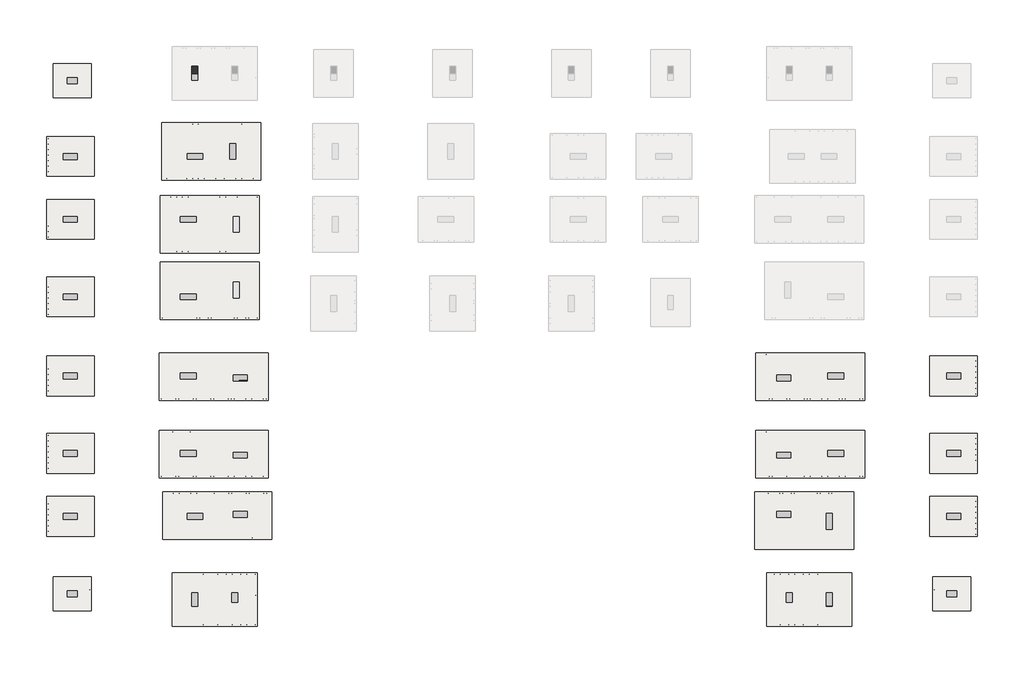
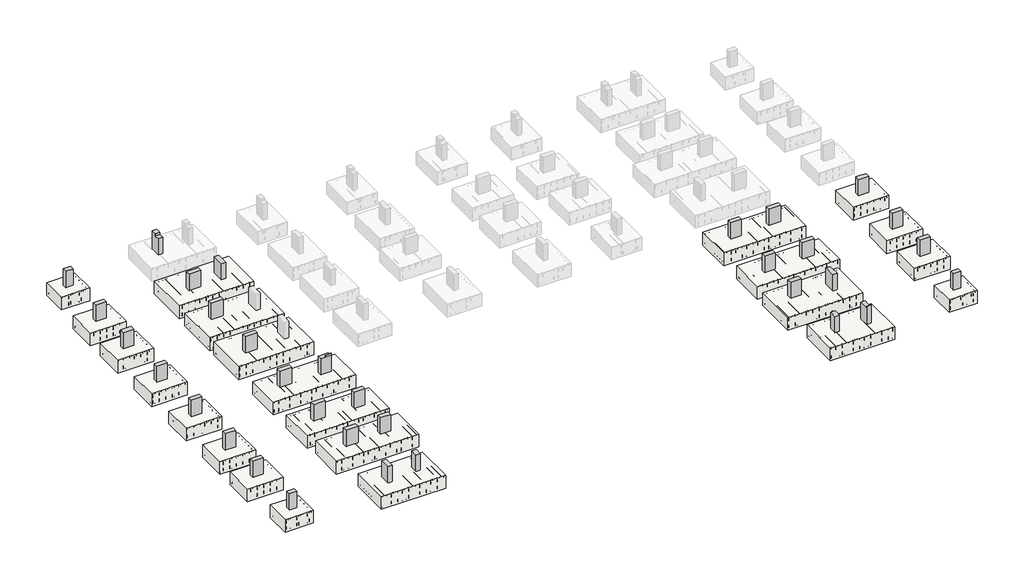
# One storey, part 1 of 21: 33 columns, 23 slabs.
"""IFC4 building model written with IfcOpenShell, lengths in millimetres."""

from ifc_helpers import new_model, si_unit, frame, origin, place, context, project, spatial, polyline, outline, extrude, faceted_brep, transform, mapped, element, save
from components import m_footing_rectangular_1900x1700x900_f1_617558a1, m_footing_rectangular_2400x2000x900_f2_ceb4d106, m_footing_rectangular_2700x4300x900_f4_c3563192, m_footing_rectangular_5000x2900x900_f5_2a8e231f, m_footing_rectangular_5500x2400x900_f6_6a8cdcd2

model = new_model("IFC4")

# Units and contexts
model_context = context("Model", 3, world=origin())
ifc_project = project(units=[si_unit("LENGTHUNIT", "METRE", prefix="MILLI")], contexts=[model_context])

# Site, building, storey
site = spatial("IfcSite", under=ifc_project)
building = spatial("IfcBuilding", under=site)
storey = spatial("IfcBuildingStorey", under=building, Elevation=-1100.0)

# Columns
placement = place(None, origin())
element("IfcColumn", 1, ObjectType="M_Concrete-Rectangular-Column : 300X500 C1", at=placement, inside=storey, context=model_context, shape_type="Brep", body=[
    faceted_brep([(-24350.8326863, 14604.1704288, -1100.0), (-23850.8326863, 14604.1704288, -1100.0), (-23850.8326863, 14304.1704288, -1100.0), (-24350.8326863, 14304.1704288, -1100.0), (-24350.8326863, 14604.1704288, 50.0), (-23850.8326863, 14604.1704288, 50.0), (-23850.8326863, 14304.1704288, 50.0), (-24150.8326863, 14304.1704288, 50.0), (-24350.8326863, 14304.1704288, 50.0)], [[[0, 1, 2, 3]], [[1, 0, 4, 5]], [[2, 1, 5, 6]], [[3, 2, 6, 7, 8]], [[0, 3, 8, 4]], [[5, 4, 8, 7, 6]]]),
])
element("IfcColumn", 2, ObjectType="M_Concrete-Rectangular-Column : 300X500 C1", at=placement, inside=storey, context=model_context, shape_type="Brep", body=[
    faceted_brep([(-24350.8326863, -11305.8295712, -1100.0), (-23850.8326863, -11305.8295712, -1100.0), (-23850.8326863, -11605.8295712, -1100.0), (-24350.8326863, -11605.8295712, -1100.0), (-24350.8326863, -11305.8295712, 50.0), (-24150.8326863, -11305.8295712, 50.0), (-23850.8326863, -11305.8295712, 50.0), (-23850.8326863, -11605.8295712, 50.0), (-24350.8326863, -11605.8295712, 50.0)], [[[0, 1, 2, 3]], [[1, 0, 4, 5, 6]], [[2, 1, 6, 7]], [[3, 2, 7, 8]], [[0, 3, 8, 4]], [[6, 5, 4, 8, 7]]]),
])
element("IfcColumn", 3, ObjectType="M_Concrete-Rectangular-Column : 300X500 C1", at=placement, inside=storey, context=model_context, shape_type="Brep", body=[
    faceted_brep([(20029.1673137, -11305.8295712, -1100.0), (20529.1673137, -11305.8295712, -1100.0), (20529.1673137, -11605.8295712, -1100.0), (20029.1673137, -11605.8295712, -1100.0), (20029.1673137, -11305.8295712, 50.0), (20329.1673137, -11305.8295712, 50.0), (20529.1673137, -11305.8295712, 50.0), (20529.1673137, -11605.8295712, 50.0), (20029.1673137, -11605.8295712, 50.0)], [[[0, 1, 2, 3]], [[1, 0, 4, 5, 6]], [[2, 1, 6, 7]], [[3, 2, 7, 8]], [[0, 3, 8, 4]], [[6, 5, 4, 8, 7]]]),
])
element("IfcColumn", 4, ObjectType="M_Concrete-Rectangular-Column : 300X500 C1", at=placement, inside=storey, context=model_context, shape_type="Brep", body=[
    faceted_brep([(11939.1673137, -11895.8295712, -1100.0), (11939.1673137, -11395.8295712, -1100.0), (12239.1673137, -11395.8295712, -1100.0), (12239.1673137, -11895.8295712, -1100.0), (11939.1673137, -11895.8295712, 50.0), (11939.1673137, -11395.8295712, 50.0), (12239.1673137, -11395.8295712, 50.0), (12239.1673137, -11695.8295712, 50.0), (12239.1673137, -11895.8295712, 50.0)], [[[0, 1, 2, 3]], [[1, 0, 4, 5]], [[2, 1, 5, 6]], [[3, 2, 6, 7, 8]], [[0, 3, 8, 4]], [[5, 4, 8, 7, 6]]]),
])
element("IfcColumn", 5, ObjectType="M_Concrete-Rectangular-Column : 300X500 C1", at=placement, inside=storey, context=model_context, shape_type="Brep", body=[
    faceted_brep([(-16061.8300669, -11895.8295712, -1100.0), (-16061.8300669, -11395.8295712, -1100.0), (-15761.8300669, -11395.8295712, -1100.0), (-15761.8300669, -11895.8295712, -1100.0), (-16061.8300669, -11895.8295712, 50.0), (-16061.8300669, -11695.8295712, 50.0), (-16061.8300669, -11395.8295712, 50.0), (-15761.8300669, -11395.8295712, 50.0), (-15761.8300669, -11895.8295712, 50.0)], [[[0, 1, 2, 3]], [[1, 0, 4, 5, 6]], [[2, 1, 6, 7]], [[3, 2, 7, 8]], [[0, 3, 8, 4]], [[6, 5, 4, 8, 7]]]),
])
element("IfcColumn", 6, ObjectType="M_Concrete-Rectangular-Column : 300X700 C2", at=placement, inside=storey, context=model_context, shape_type="Brep", body=[
    faceted_brep([(-17760.8326863, 15184.1704288, -1100.0), (-17760.8326863, 14484.1704288, -1100.0), (-18060.8326863, 14484.1704288, -1100.0), (-18060.8326863, 15184.1704288, -1100.0), (-17760.8326863, 15184.1704288, 200.0), (-17760.8326863, 14806.5875097, 200.0), (-17760.8326863, 14806.5875097, 50.0), (-17760.8326863, 14484.1704288, 50.0), (-18060.8326863, 14484.1704288, 50.0), (-18060.8326863, 14806.3616842, 50.0), (-18060.8326863, 14806.3616842, 200.0), (-18060.8326863, 15184.1704288, 200.0), (-18054.3658896, 14806.5875097, 200.0), (-18054.3658896, 14806.5875097, 50.0)], [[[0, 1, 2, 3]], [[1, 0, 4, 5, 6, 7]], [[2, 1, 7, 8]], [[3, 2, 8, 9, 10, 11]], [[0, 3, 11, 4]], [[4, 11, 10, 12, 5]], [[6, 13, 9, 8, 7]], [[13, 12, 10, 9]], [[12, 13, 6, 5]]]),
])
element("IfcColumn", 7, ObjectType="M_Concrete-Rectangular-Column : 300X700 C2", at=placement, inside=storey, context=model_context, shape_type="Brep", body=[
    faceted_brep([(-24550.8326863, 7604.1704288, -1100.0), (-23850.8326863, 7604.1704288, -1100.0), (-23850.8326863, 7304.1704288, -1100.0), (-24550.8326863, 7304.1704288, -1100.0), (-24550.8326863, 7604.1704288, 50.0), (-24150.8326863, 7604.1704288, 50.0), (-23850.8326863, 7604.1704288, 50.0), (-23850.8326863, 7604.1704288, -400.0), (-23850.8326863, 7304.1704288, 50.0), (-23850.8326863, 7304.1704288, -400.0), (-24150.8326863, 7304.1704288, 50.0), (-24550.8326863, 7304.1704288, 50.0)], [[[0, 1, 2, 3]], [[1, 0, 4, 5, 6, 7]], [[2, 1, 7, 6, 8, 9]], [[3, 2, 9, 8, 10, 11]], [[0, 3, 11, 4]], [[6, 5, 4, 11, 10, 8]]]),
])
element("IfcColumn", 8, ObjectType="M_Concrete-Rectangular-Column : 300X700 C2", at=placement, inside=storey, context=model_context, shape_type="Brep", body=[
    faceted_brep([(-24550.8326863, 3694.1704288, -1100.0), (-23850.8326863, 3694.1704288, -1100.0), (-23850.8326863, 3394.1704288, -1100.0), (-24550.8326863, 3394.1704288, -1100.0), (-24550.8326863, 3694.1704288, 50.0), (-24150.8326863, 3694.1704288, 50.0), (-23850.8326863, 3694.1704288, 50.0), (-23850.8326863, 3694.1704288, -400.0), (-23850.8326863, 3394.1704288, 50.0), (-23850.8326863, 3394.1704288, -400.0), (-24150.8326863, 3394.1704288, 50.0), (-24550.8326863, 3394.1704288, 50.0)], [[[0, 1, 2, 3]], [[1, 0, 4, 5, 6, 7]], [[2, 1, 7, 6, 8, 9]], [[3, 2, 9, 8, 10, 11]], [[0, 3, 11, 4]], [[6, 5, 4, 11, 10, 8]]]),
])
element("IfcColumn", 9, ObjectType="M_Concrete-Rectangular-Column : 300X700 C2", at=placement, inside=storey, context=model_context, shape_type="Brep", body=[
    faceted_brep([(-24550.8326863, -305.8295712, -1100.0), (-23850.8326863, -305.8295712, -1100.0), (-23850.8326863, -605.8295712, -1100.0), (-24550.8326863, -605.8295712, -1100.0), (-24550.8326863, -305.8295712, 50.0), (-24150.8326863, -305.8295712, 50.0), (-23850.8326863, -305.8295712, 50.0), (-23850.8326863, -305.8295712, -400.0), (-23850.8326863, -605.8295712, 50.0), (-23850.8326863, -605.8295712, -400.0), (-24150.8326863, -605.8295712, 50.0), (-24550.8326863, -605.8295712, 50.0)], [[[0, 1, 2, 3]], [[1, 0, 4, 5, 6, 7]], [[2, 1, 7, 6, 8, 9]], [[3, 2, 9, 8, 10, 11]], [[0, 3, 11, 4]], [[6, 5, 4, 11, 10, 8]]]),
])
element("IfcColumn", 10, ObjectType="M_Concrete-Rectangular-Column : 300X700 C2", at=placement, inside=storey, context=model_context, shape_type="Brep", body=[
    faceted_brep([(-24550.8326863, -4215.8295712, -1100.0), (-23850.8326863, -4215.8295712, -1100.0), (-23850.8326863, -4515.8295712, -1100.0), (-24550.8326863, -4515.8295712, -1100.0), (-24550.8326863, -4215.8295712, 50.0), (-24150.8326863, -4215.8295712, 50.0), (-23850.8326863, -4215.8295712, 50.0), (-23850.8326863, -4215.8295712, -400.0), (-23850.8326863, -4515.8295712, 50.0), (-23850.8326863, -4515.8295712, -400.0), (-24150.8326863, -4515.8295712, 50.0), (-24550.8326863, -4515.8295712, 50.0)], [[[0, 1, 2, 3]], [[1, 0, 4, 5, 6, 7]], [[2, 1, 7, 6, 8, 9]], [[3, 2, 9, 8, 10, 11]], [[0, 3, 11, 4]], [[6, 5, 4, 11, 10, 8]]]),
])
element("IfcColumn", 11, ObjectType="M_Concrete-Rectangular-Column : 300X700 C2", at=placement, inside=storey, context=model_context, shape_type="Brep", body=[
    faceted_brep([(-24550.8326863, -7395.8295712, -1100.0), (-23850.8326863, -7395.8295712, -1100.0), (-23850.8326863, -7695.8295712, -1100.0), (-24550.8326863, -7695.8295712, -1100.0), (-24550.8326863, -7395.8295712, 50.0), (-24150.8326863, -7395.8295712, 50.0), (-23850.8326863, -7395.8295712, 50.0), (-23850.8326863, -7395.8295712, -400.0), (-23850.8326863, -7695.8295712, 50.0), (-23850.8326863, -7695.8295712, -400.0), (-24150.8326863, -7695.8295712, 50.0), (-24550.8326863, -7695.8295712, 50.0)], [[[0, 1, 2, 3]], [[1, 0, 4, 5, 6, 7]], [[2, 1, 7, 6, 8, 9]], [[3, 2, 9, 8, 10, 11]], [[0, 3, 11, 4]], [[6, 5, 4, 11, 10, 8]]]),
])
element("IfcColumn", 12, ObjectType="M_Concrete-Rectangular-Column : 300X700 C2", at=placement, inside=storey, context=model_context, shape_type="Brep", body=[
    faceted_brep([(-18060.8326863, -12095.8295712, -1100.0), (-18060.8326863, -11395.8295712, -1100.0), (-17760.8326863, -11395.8295712, -1100.0), (-17760.8326863, -12095.8295712, -1100.0), (-18060.8326863, -12095.8295712, 50.0), (-18060.8326863, -11691.586009, 50.0), (-18060.8326863, -11395.8295712, 50.0), (-17760.8326863, -11395.8295712, 50.0), (-17760.8326863, -11695.8295712, 50.0), (-17760.8326863, -12095.8295712, 50.0)], [[[0, 1, 2, 3]], [[1, 0, 4, 5, 6]], [[2, 1, 6, 7]], [[3, 2, 7, 8, 9]], [[0, 3, 9, 4]], [[6, 5, 4, 9, 8, 7]]]),
])
element("IfcColumn", 13, ObjectType="M_Concrete-Rectangular-Column : 300X700 C2", at=placement, inside=storey, context=model_context, shape_type="Brep", body=[
    faceted_brep([(-15270.8326863, -7605.8295712, -1100.0), (-15970.8326863, -7605.8295712, -1100.0), (-15970.8326863, -7305.8295712, -1100.0), (-15270.8326863, -7305.8295712, -1100.0), (-15270.8326863, -7605.8295712, 50.0), (-15670.8326863, -7605.8295712, 50.0), (-15970.8326863, -7605.8295712, 50.0), (-15970.8326863, -7305.8295712, 50.0), (-15670.8326863, -7305.8295712, 50.0), (-15270.8326863, -7305.8295712, 50.0)], [[[0, 1, 2, 3]], [[1, 0, 4, 5, 6]], [[2, 1, 6, 7]], [[3, 2, 7, 8, 9]], [[0, 3, 9, 4]], [[6, 5, 4, 9, 8, 7]]]),
])
element("IfcColumn", 14, ObjectType="M_Concrete-Rectangular-Column : 300X700 C2", at=placement, inside=storey, context=model_context, shape_type="Brep", body=[
    faceted_brep([(-15270.8326863, -4605.8295712, -1100.0), (-15970.8326863, -4605.8295712, -1100.0), (-15970.8326863, -4305.8295712, -1100.0), (-15270.8326863, -4305.8295712, -1100.0), (-15270.8326863, -4605.8295712, 50.0), (-15670.8326863, -4605.8295712, 50.0), (-15970.8326863, -4605.8295712, 50.0), (-15970.8326863, -4605.8295712, -400.0), (-15970.8326863, -4305.8295712, 50.0), (-15970.8326863, -4305.8295712, -400.0), (-15670.8326863, -4305.8295712, 50.0), (-15270.8326863, -4305.8295712, 50.0)], [[[0, 1, 2, 3]], [[1, 0, 4, 5, 6, 7]], [[2, 1, 7, 6, 8, 9]], [[3, 2, 9, 8, 10, 11]], [[0, 3, 11, 4]], [[6, 5, 4, 11, 10, 8]]]),
])
element("IfcColumn", 15, ObjectType="M_Concrete-Rectangular-Column : 300X700 C2", at=placement, inside=storey, context=model_context, shape_type="Brep", body=[
    faceted_brep([(-15270.8326863, -695.8295712, -1100.0), (-15970.8326863, -695.8295712, -1100.0), (-15970.8326863, -395.8295712, -1100.0), (-15270.8326863, -395.8295712, -1100.0), (-15270.8326863, -695.8295712, 200.0), (-15670.8326863, -695.8295712, 200.0), (-15670.8326863, -695.8295712, 50.0), (-15970.8326863, -695.8295712, 50.0), (-15970.8326863, -695.8295712, -400.0), (-15970.8326863, -395.8295712, 50.0), (-15970.8326863, -395.8295712, -400.0), (-15270.8326863, -395.8295712, 50.0), (-15270.8326863, -693.8316044, 50.0), (-15270.8326863, -693.8316044, 200.0), (-15670.8326863, -693.8316044, 200.0), (-15670.8326863, -693.8316044, 50.0)], [[[0, 1, 2, 3]], [[1, 0, 4, 5, 6, 7, 8]], [[2, 1, 8, 7, 9, 10]], [[3, 2, 10, 9, 11]], [[0, 3, 11, 12, 13, 4]], [[4, 13, 14, 5]], [[15, 12, 11, 9, 7, 6]], [[12, 15, 14, 13]], [[14, 15, 6, 5]]]),
])
element("IfcColumn", 16, ObjectType="M_Concrete-Rectangular-Column : 300X700 C2", at=placement, inside=storey, context=model_context, shape_type="Brep", body=[
    faceted_brep([(20029.1673137, -305.8295712, -1100.0), (20729.1673137, -305.8295712, -1100.0), (20729.1673137, -605.8295712, -1100.0), (20029.1673137, -605.8295712, -1100.0), (20029.1673137, -305.8295712, -400.0), (20029.1673137, -305.8295712, 50.0), (20329.1673137, -305.8295712, 50.0), (20729.1673137, -305.8295712, 50.0), (20729.1673137, -605.8295712, 50.0), (20329.1673137, -605.8295712, 50.0), (20029.1673137, -605.8295712, 50.0), (20029.1673137, -605.8295712, -400.0)], [[[0, 1, 2, 3]], [[1, 0, 4, 5, 6, 7]], [[2, 1, 7, 8]], [[3, 2, 8, 9, 10, 11]], [[0, 3, 11, 10, 5, 4]], [[7, 6, 5, 10, 9, 8]]]),
])
element("IfcColumn", 17, ObjectType="M_Concrete-Rectangular-Column : 300X700 C2", at=placement, inside=storey, context=model_context, shape_type="Brep", body=[
    faceted_brep([(20029.1673137, -4215.8295712, -1100.0), (20729.1673137, -4215.8295712, -1100.0), (20729.1673137, -4515.8295712, -1100.0), (20029.1673137, -4515.8295712, -1100.0), (20029.1673137, -4215.8295712, -400.0), (20029.1673137, -4215.8295712, 50.0), (20329.1673137, -4215.8295712, 50.0), (20729.1673137, -4215.8295712, 50.0), (20729.1673137, -4515.8295712, 50.0), (20329.1673137, -4515.8295712, 50.0), (20029.1673137, -4515.8295712, 50.0), (20029.1673137, -4515.8295712, -400.0)], [[[0, 1, 2, 3]], [[1, 0, 4, 5, 6, 7]], [[2, 1, 7, 8]], [[3, 2, 8, 9, 10, 11]], [[0, 3, 11, 10, 5, 4]], [[7, 6, 5, 10, 9, 8]]]),
])
element("IfcColumn", 18, ObjectType="M_Concrete-Rectangular-Column : 300X700 C2", at=placement, inside=storey, context=model_context, shape_type="Brep", body=[
    faceted_brep([(20029.1673137, -7395.8295712, -1100.0), (20729.1673137, -7395.8295712, -1100.0), (20729.1673137, -7695.8295712, -1100.0), (20029.1673137, -7695.8295712, -1100.0), (20029.1673137, -7395.8295712, -400.0), (20029.1673137, -7395.8295712, 50.0), (20329.1673137, -7395.8295712, 50.0), (20729.1673137, -7395.8295712, 50.0), (20729.1673137, -7695.8295712, 50.0), (20329.1673137, -7695.8295712, 50.0), (20029.1673137, -7695.8295712, 50.0), (20029.1673137, -7695.8295712, -400.0)], [[[0, 1, 2, 3]], [[1, 0, 4, 5, 6, 7]], [[2, 1, 7, 8]], [[3, 2, 8, 9, 10, 11]], [[0, 3, 11, 10, 5, 4]], [[7, 6, 5, 10, 9, 8]]]),
])
element("IfcColumn", 19, ObjectType="M_Concrete-Rectangular-Column : 300X700 C2", at=placement, inside=storey, context=model_context, shape_type="Brep", body=[
    faceted_brep([(13939.1673137, -12095.8295712, -1100.0), (13939.1673137, -11395.8295712, -1100.0), (14239.1673137, -11395.8295712, -1100.0), (14239.1673137, -12095.8295712, -1100.0), (13939.1673137, -12095.8295712, 200.0), (13939.1673137, -12095.6219296, 200.0), (13939.1673137, -12095.6219296, 50.0), (13939.1673137, -11695.8295712, 50.0), (13939.1673137, -11395.8295712, 50.0), (14239.1673137, -11395.8295712, 50.0), (14239.1673137, -11715.6219296, 50.0), (14239.1673137, -12095.6219296, 50.0), (14239.1673137, -12095.6219296, 200.0), (14239.1673137, -12095.8295712, 200.0)], [[[0, 1, 2, 3]], [[1, 0, 4, 5, 6, 7, 8]], [[2, 1, 8, 9]], [[3, 2, 9, 10, 11, 12, 13]], [[0, 3, 13, 4]], [[4, 13, 12, 5]], [[6, 11, 10, 9, 8, 7]], [[11, 6, 5, 12]]]),
])
element("IfcColumn", 20, ObjectType="M_Concrete-Rectangular-Column : 300X700 C2", at=placement, inside=storey, context=model_context, shape_type="Brep", body=[
    faceted_brep([(11449.1673137, -7305.8295712, -1100.0), (12149.1673137, -7305.8295712, -1100.0), (12149.1673137, -7605.8295712, -1100.0), (11449.1673137, -7605.8295712, -1100.0), (11449.1673137, -7305.8295712, 50.0), (11849.1673137, -7305.8295712, 50.0), (12149.1673137, -7305.8295712, 50.0), (12149.1673137, -7605.8295712, 50.0), (11449.1673137, -7605.8295712, 50.0)], [[[0, 1, 2, 3]], [[1, 0, 4, 5, 6]], [[2, 1, 6, 7]], [[3, 2, 7, 8]], [[0, 3, 8, 4]], [[6, 5, 4, 8, 7]]]),
])
element("IfcColumn", 21, ObjectType="M_Concrete-Rectangular-Column : 300X700 C2", at=placement, inside=storey, context=model_context, shape_type="Brep", body=[
    faceted_brep([(11449.1673137, -4305.8295712, -1100.0), (12149.1673137, -4305.8295712, -1100.0), (12149.1673137, -4605.8295712, -1100.0), (11449.1673137, -4605.8295712, -1100.0), (11449.1673137, -4305.8295712, 50.0), (11849.1673137, -4305.8295712, 50.0), (12149.1673137, -4305.8295712, 50.0), (12149.1673137, -4305.8295712, -400.0), (12149.1673137, -4605.8295712, 50.0), (12149.1673137, -4605.8295712, -400.0), (11849.1673137, -4605.8295712, 50.0), (11449.1673137, -4605.8295712, 50.0)], [[[0, 1, 2, 3]], [[1, 0, 4, 5, 6, 7]], [[2, 1, 7, 6, 8, 9]], [[3, 2, 9, 8, 10, 11]], [[0, 3, 11, 4]], [[6, 5, 4, 11, 10, 8]]]),
])
element("IfcColumn", 22, ObjectType="M_Concrete-Rectangular-Column : 300X700 C2", at=placement, inside=storey, context=model_context, shape_type="Brep", body=[
    faceted_brep([(11449.1673137, -395.8295712, -1100.0), (12149.1673137, -395.8295712, -1100.0), (12149.1673137, -695.8295712, -1100.0), (11449.1673137, -695.8295712, -1100.0), (11449.1673137, -395.8295712, 50.0), (11849.1673137, -395.8295712, 50.0), (12149.1673137, -395.8295712, 50.0), (12149.1673137, -395.8295712, -400.0), (12149.1673137, -695.8295712, 50.0), (12149.1673137, -695.8295712, -400.0), (11849.1673137, -695.8295712, 50.0), (11449.1673137, -695.8295712, 50.0)], [[[0, 1, 2, 3]], [[1, 0, 4, 5, 6, 7]], [[2, 1, 7, 6, 8, 9]], [[3, 2, 9, 8, 10, 11]], [[0, 3, 11, 4]], [[6, 5, 4, 11, 10, 8]]]),
])
element("IfcColumn", 23, ObjectType="M_Concrete-Rectangular-Column : 300X700 C2", at=placement, inside=storey, context=model_context, shape_type="Brep", body=[
    faceted_brep([(-24550.8326863, 10779.2254822, -1100.0), (-23850.8326863, 10779.2254822, -1100.0), (-23850.8326863, 10479.2254822, -1100.0), (-24550.8326863, 10479.2254822, -1100.0), (-24550.8326863, 10779.2254822, 50.0), (-24150.8326863, 10779.2254822, 50.0), (-23850.8326863, 10779.2254822, 50.0), (-23850.8326863, 10779.2254822, -400.0), (-23850.8326863, 10479.2254822, 50.0), (-23850.8326863, 10479.2254822, -400.0), (-24150.8326863, 10479.2254822, 50.0), (-24550.8326863, 10479.2254822, 50.0)], [[[0, 1, 2, 3]], [[1, 0, 4, 5, 6, 7]], [[2, 1, 7, 6, 8, 9]], [[3, 2, 9, 8, 10, 11]], [[0, 3, 11, 4]], [[6, 5, 4, 11, 10, 8]]]),
])
element("IfcColumn", 24, ObjectType="M_Concrete-Rectangular-Column : 300X800 C3", at=placement, inside=storey, context=model_context, shape_type="SweptSolid", body=[
    extrude(outline(polyline([(-18310.8326863, -7395.8295712), (-17510.8326863, -7395.8295712), (-17510.8326863, -7695.8295712), (-18310.8326863, -7695.8295712), (-18310.8326863, -7395.8295712)])), frame((0.0, 0.0, -1100.0), z_axis=(0.0, 0.0, 1.0), x_axis=(1.0, 0.0, 0.0)), (0.0, 0.0, 1.0), 1150.0),
])
element("IfcColumn", 25, ObjectType="M_Concrete-Rectangular-Column : 300X800 C3", at=placement, inside=storey, context=model_context, shape_type="Brep", body=[
    faceted_brep([(-18650.8326863, -4215.8295712, -1100.0), (-17850.8326863, -4215.8295712, -1100.0), (-17850.8326863, -4515.8295712, -1100.0), (-18650.8326863, -4515.8295712, -1100.0), (-18650.8326863, -4215.8295712, 50.0), (-18150.8326863, -4215.8295712, 50.0), (-17850.8326863, -4215.8295712, 50.0), (-17850.8326863, -4215.8295712, -400.0), (-17850.8326863, -4515.8295712, 50.0), (-17850.8326863, -4515.8295712, -400.0), (-18150.8326863, -4515.8295712, 50.0), (-18650.8326863, -4515.8295712, 50.0)], [[[0, 1, 2, 3]], [[1, 0, 4, 5, 6, 7]], [[2, 1, 7, 6, 8, 9]], [[3, 2, 9, 8, 10, 11]], [[0, 3, 11, 4]], [[6, 5, 4, 11, 10, 8]]]),
])
element("IfcColumn", 26, ObjectType="M_Concrete-Rectangular-Column : 300X800 C3", at=placement, inside=storey, context=model_context, shape_type="Brep", body=[
    faceted_brep([(-18650.8326863, -305.8295712, -1100.0), (-17850.8326863, -305.8295712, -1100.0), (-17850.8326863, -605.8295712, -1100.0), (-18650.8326863, -605.8295712, -1100.0), (-18650.8326863, -305.8295712, -400.0), (-18650.8326863, -305.8295712, 50.0), (-18150.8326863, -305.8295712, 50.0), (-17850.8326863, -305.8295712, 50.0), (-17850.8326863, -305.8295712, -400.0), (-17850.8326863, -605.8295712, 50.0), (-17850.8326863, -605.8295712, -400.0), (-18150.8326863, -605.8295712, 50.0), (-18650.8326863, -605.8295712, 50.0), (-18650.8326863, -605.8295712, -400.0)], [[[0, 1, 2, 3]], [[1, 0, 4, 5, 6, 7, 8]], [[2, 1, 8, 7, 9, 10]], [[3, 2, 10, 9, 11, 12, 13]], [[0, 3, 13, 12, 5, 4]], [[7, 6, 5, 12, 11, 9]]]),
])
element("IfcColumn", 27, ObjectType="M_Concrete-Rectangular-Column : 300X800 C3", at=placement, inside=storey, context=model_context, shape_type="Brep", body=[
    faceted_brep([(-18650.8326863, 3694.1704288, -1100.0), (-17850.8326863, 3694.1704288, -1100.0), (-17850.8326863, 3394.1704288, -1100.0), (-18650.8326863, 3394.1704288, -1100.0), (-18650.8326863, 3694.1704288, 50.0), (-18150.8326863, 3694.1704288, 50.0), (-17850.8326863, 3694.1704288, 50.0), (-17850.8326863, 3694.1704288, -400.0), (-17850.8326863, 3394.1704288, 50.0), (-17850.8326863, 3394.1704288, -400.0), (-18150.8326863, 3394.1704288, 50.0), (-18650.8326863, 3394.1704288, 50.0)], [[[0, 1, 2, 3]], [[1, 0, 4, 5, 6, 7]], [[2, 1, 7, 6, 8, 9]], [[3, 2, 9, 8, 10, 11]], [[0, 3, 11, 4]], [[6, 5, 4, 11, 10, 8]]]),
])
element("IfcColumn", 28, ObjectType="M_Concrete-Rectangular-Column : 300X800 C3", at=placement, inside=storey, context=model_context, shape_type="Brep", body=[
    faceted_brep([(-18650.8326863, 7604.1704288, -1100.0), (-17850.8326863, 7604.1704288, -1100.0), (-17850.8326863, 7304.1704288, -1100.0), (-18650.8326863, 7304.1704288, -1100.0), (-18650.8326863, 7604.1704288, -400.0), (-18650.8326863, 7604.1704288, 50.0), (-18150.8326863, 7604.1704288, 50.0), (-17850.8326863, 7604.1704288, 50.0), (-17850.8326863, 7604.1704288, -400.0), (-17850.8326863, 7304.1704288, 50.0), (-17850.8326863, 7304.1704288, -400.0), (-18150.8326863, 7304.1704288, 50.0), (-18650.8326863, 7304.1704288, 50.0), (-18650.8326863, 7304.1704288, -400.0)], [[[0, 1, 2, 3]], [[1, 0, 4, 5, 6, 7, 8]], [[2, 1, 8, 7, 9, 10]], [[3, 2, 10, 9, 11, 12, 13]], [[0, 3, 13, 12, 5, 4]], [[7, 6, 5, 12, 11, 9]]]),
])
element("IfcColumn", 29, ObjectType="M_Concrete-Rectangular-Column : 300X800 C3", at=placement, inside=storey, context=model_context, shape_type="Brep", body=[
    faceted_brep([(-16150.8326863, 10484.1704288, -1100.0), (-16150.8326863, 11284.1704288, -1100.0), (-15850.8326863, 11284.1704288, -1100.0), (-15850.8326863, 10484.1704288, -1100.0), (-16150.8326863, 10484.1704288, -400.0), (-16150.8326863, 10484.1704288, 50.0), (-16150.8326863, 10784.1704288, 50.0), (-16150.8326863, 11284.1704288, 50.0), (-15850.8326863, 11284.1704288, 50.0), (-15850.8326863, 10784.1704288, 50.0), (-15850.8326863, 10638.2890293, 50.0), (-15850.8326863, 10484.1704288, 50.0)], [[[0, 1, 2, 3]], [[1, 0, 4, 5, 6, 7]], [[2, 1, 7, 8]], [[3, 2, 8, 9, 10, 11]], [[0, 3, 11, 5, 4]], [[7, 6, 5, 11, 10, 9, 8]]]),
])
element("IfcColumn", 30, ObjectType="M_Concrete-Rectangular-Column : 300X800 C3", at=placement, inside=storey, context=model_context, shape_type="Brep", body=[
    faceted_brep([(-17510.8326863, 10484.1704288, -1100.0), (-18310.8326863, 10484.1704288, -1100.0), (-18310.8326863, 10784.1704288, -1100.0), (-17510.8326863, 10784.1704288, -1100.0), (-17510.8326863, 10484.1704288, -400.0), (-17510.8326863, 10484.1704288, 50.0), (-18310.8326863, 10484.1704288, 50.0), (-18310.8326863, 10484.1704288, -400.0), (-18310.8326863, 10784.1704288, 50.0), (-18310.8326863, 10784.1704288, -400.0), (-17510.8326863, 10784.1704288, 50.0), (-17510.8326863, 10784.1704288, -400.0)], [[[0, 1, 2, 3]], [[1, 0, 4, 5, 6, 7]], [[2, 1, 7, 6, 8, 9]], [[3, 2, 9, 8, 10, 11]], [[0, 3, 11, 10, 5, 4]], [[6, 5, 10, 8]]]),
])
element("IfcColumn", 31, ObjectType="M_Concrete-Rectangular-Column : 300X800 C3", at=placement, inside=storey, context=model_context, shape_type="Brep", body=[
    faceted_brep([(14029.1673137, -305.8295712, -1100.0), (14829.1673137, -305.8295712, -1100.0), (14829.1673137, -605.8295712, -1100.0), (14029.1673137, -605.8295712, -1100.0), (14029.1673137, -305.8295712, -400.0), (14029.1673137, -305.8295712, 50.0), (14329.1673137, -305.8295712, 50.0), (14829.1673137, -305.8295712, 50.0), (14829.1673137, -605.8295712, 50.0), (14329.1673137, -605.8295712, 50.0), (14029.1673137, -605.8295712, 50.0), (14029.1673137, -605.8295712, -400.0)], [[[0, 1, 2, 3]], [[1, 0, 4, 5, 6, 7]], [[2, 1, 7, 8]], [[3, 2, 8, 9, 10, 11]], [[0, 3, 11, 10, 5, 4]], [[7, 6, 5, 10, 9, 8]]]),
])
element("IfcColumn", 32, ObjectType="M_Concrete-Rectangular-Column : 300X800 C3", at=placement, inside=storey, context=model_context, shape_type="SweptSolid", body=[
    extrude(outline(polyline([(14829.1673137, -4515.8295712), (14029.1673137, -4515.8295712), (14029.1673137, -4215.8295712), (14829.1673137, -4215.8295712), (14829.1673137, -4515.8295712)])), frame((0.0, 0.0, -1100.0), z_axis=(0.0, 0.0, 1.0), x_axis=(1.0, 0.0, 0.0)), (0.0, 0.0, 1.0), 1150.0),
])
element("IfcColumn", 33, ObjectType="M_Concrete-Rectangular-Column : 300X800 C3", at=placement, inside=storey, context=model_context, shape_type="SweptSolid", body=[
    extrude(outline(polyline([(14239.1673137, -7395.8295712), (14239.1673137, -8195.8295712), (13939.1673137, -8195.8295712), (13939.1673137, -7395.8295712), (14239.1673137, -7395.8295712)])), frame((0.0, 0.0, -1100.0), z_axis=(0.0, 0.0, 1.0), x_axis=(1.0, 0.0, 0.0)), (0.0, 0.0, 1.0), 1150.0),
])

# Slabs
element("IfcSlab", 34, ObjectType="M_Footing-Rectangular : 1900X1700X900 F1", at=placement, inside=storey, context=model_context, shape_type="SweptSolid", body=[
    extrude(outline(polyline([(-23150.8326863, -10605.8295712), (-23150.8326863, -12305.8295712), (-25050.8326863, -12305.8295712), (-25050.8326863, -10605.8295712), (-23150.8326863, -10605.8295712)])), frame((0.0, 0.0, -2000.0), z_axis=(0.0, 0.0, 1.0), x_axis=(1.0, 0.0, 0.0)), (0.0, 0.0, 1.0), 900.0),
])
m_footing_rectangular_1900x1700x900_f1_shape = m_footing_rectangular_1900x1700x900_f1_617558a1(model_context)
element("IfcSlab", 35, ObjectType="M_Footing-Rectangular : 1900X1700X900 F1", at=placement, inside=storey, context=model_context, shape_type="MappedRepresentation", body=[
    mapped(m_footing_rectangular_1900x1700x900_f1_shape, transform((-24100.8326863, 14454.1704288, -1100.0), x_axis=(1.0, 0.0, 0.0), y_axis=(0.0, 1.0, 0.0), z_axis=(0.0, 0.0, 1.0))),
])
element("IfcSlab", 36, ObjectType="M_Footing-Rectangular : 1900X1700X900 F1", at=placement, inside=storey, context=model_context, shape_type="MappedRepresentation", body=[
    mapped(m_footing_rectangular_1900x1700x900_f1_shape, transform((20279.1673137, -11455.8295712, -1100.0), x_axis=(1.0, 0.0, 0.0), y_axis=(0.0, 1.0, 0.0), z_axis=(0.0, 0.0, 1.0))),
])
m_footing_rectangular_2400x2000x900_f2_shape = m_footing_rectangular_2400x2000x900_f2_ceb4d106(model_context)
element("IfcSlab", 37, ObjectType="M_Footing-Rectangular : 2400X2000X900 F2", at=placement, inside=storey, context=model_context, shape_type="MappedRepresentation", body=[
    mapped(m_footing_rectangular_2400x2000x900_f2_shape, transform((-24201.1351198, 10629.2254822, -1100.0), x_axis=(1.0, 0.0, 0.0), y_axis=(0.0, 1.0, 0.0), z_axis=(0.0, 0.0, 1.0))),
])
element("IfcSlab", 38, ObjectType="M_Footing-Rectangular : 2400X2000X900 F2", at=placement, inside=storey, context=model_context, shape_type="MappedRepresentation", body=[
    mapped(m_footing_rectangular_2400x2000x900_f2_shape, transform((-24201.1351198, 7454.1704288, -1100.0), x_axis=(1.0, 0.0, 0.0), y_axis=(0.0, 1.0, 0.0), z_axis=(0.0, 0.0, 1.0))),
])
element("IfcSlab", 39, ObjectType="M_Footing-Rectangular : 2400X2000X900 F2", at=placement, inside=storey, context=model_context, shape_type="MappedRepresentation", body=[
    mapped(m_footing_rectangular_2400x2000x900_f2_shape, transform((-24201.1351198, 3544.1704288, -1100.0), x_axis=(1.0, 0.0, 0.0), y_axis=(0.0, 1.0, 0.0), z_axis=(0.0, 0.0, 1.0))),
])
element("IfcSlab", 40, ObjectType="M_Footing-Rectangular : 2400X2000X900 F2", at=placement, inside=storey, context=model_context, shape_type="MappedRepresentation", body=[
    mapped(m_footing_rectangular_2400x2000x900_f2_shape, transform((-24201.1351198, -455.8295712, -1100.0), x_axis=(1.0, 0.0, 0.0), y_axis=(0.0, 1.0, 0.0), z_axis=(0.0, 0.0, 1.0))),
])
element("IfcSlab", 41, ObjectType="M_Footing-Rectangular : 2400X2000X900 F2", at=placement, inside=storey, context=model_context, shape_type="MappedRepresentation", body=[
    mapped(m_footing_rectangular_2400x2000x900_f2_shape, transform((-24201.1351198, -4365.8295712, -1100.0), x_axis=(1.0, 0.0, 0.0), y_axis=(0.0, 1.0, 0.0), z_axis=(0.0, 0.0, 1.0))),
])
element("IfcSlab", 42, ObjectType="M_Footing-Rectangular : 2400X2000X900 F2", at=placement, inside=storey, context=model_context, shape_type="MappedRepresentation", body=[
    mapped(m_footing_rectangular_2400x2000x900_f2_shape, transform((-24201.1351198, -7545.8295712, -1100.0), x_axis=(1.0, 0.0, 0.0), y_axis=(0.0, 1.0, 0.0), z_axis=(0.0, 0.0, 1.0))),
])
element("IfcSlab", 43, ObjectType="M_Footing-Rectangular : 2400X2000X900 F2", at=placement, inside=storey, context=model_context, shape_type="MappedRepresentation", body=[
    mapped(m_footing_rectangular_2400x2000x900_f2_shape, transform((20379.1673659, -455.8295712, -1100.0), x_axis=(-1.0, 0.0, 0.0), y_axis=(0.0, -1.0, 0.0), z_axis=(0.0, 0.0, 1.0))),
])
element("IfcSlab", 44, ObjectType="M_Footing-Rectangular : 2400X2000X900 F2", at=placement, inside=storey, context=model_context, shape_type="MappedRepresentation", body=[
    mapped(m_footing_rectangular_2400x2000x900_f2_shape, transform((20379.1673659, -4365.8295712, -1100.0), x_axis=(-1.0, 0.0, 0.0), y_axis=(0.0, -1.0, 0.0), z_axis=(0.0, 0.0, 1.0))),
])
element("IfcSlab", 45, ObjectType="M_Footing-Rectangular : 2400X2000X900 F2", at=placement, inside=storey, context=model_context, shape_type="MappedRepresentation", body=[
    mapped(m_footing_rectangular_2400x2000x900_f2_shape, transform((20379.1673659, -7545.8295712, -1100.0), x_axis=(-1.0, 0.0, 0.0), y_axis=(0.0, -1.0, 0.0), z_axis=(0.0, 0.0, 1.0))),
])
element("IfcSlab", 46, ObjectType="M_Footing-Rectangular : 2700X4300X900 F4", at=placement, inside=storey, context=model_context, shape_type="SweptSolid", body=[
    extrude(outline(polyline([(-19060.8326863, -10395.8295712), (-14760.8326863, -10395.8295712), (-14760.8326863, -13095.8295712), (-19060.8326863, -13095.8295712), (-19060.8326863, -10395.8295712)])), frame((0.0, 0.0, -2000.0), z_axis=(0.0, 0.0, 1.0), x_axis=(1.0, 0.0, 0.0)), (0.0, 0.0, 1.0), 900.0),
])
m_footing_rectangular_2700x4300x900_f4_shape = m_footing_rectangular_2700x4300x900_f4_c3563192(model_context)
element("IfcSlab", 47, ObjectType="M_Footing-Rectangular : 2700X4300X900 F4", at=placement, inside=storey, context=model_context, shape_type="MappedRepresentation", body=[
    mapped(m_footing_rectangular_2700x4300x900_f4_shape, transform((13089.1673137, -11745.8295712, -1100.0), x_axis=(0.0, 1.0, 0.0), y_axis=(-1.0, 0.0, 0.0), z_axis=(0.0, 0.0, 1.0))),
])
m_footing_rectangular_5000x2900x900_f5_shape = m_footing_rectangular_5000x2900x900_f5_2a8e231f(model_context)
element("IfcSlab", 48, ObjectType="M_Footing-Rectangular : 5000X2900X900 F5", at=placement, inside=storey, context=model_context, shape_type="MappedRepresentation", body=[
    mapped(m_footing_rectangular_5000x2900x900_f5_shape, transform((-17080.8326863, 10884.1978555, -1100.0), x_axis=(0.0, 1.0, 0.0), y_axis=(-1.0, 0.0, 0.0), z_axis=(0.0, 0.0, 1.0))),
])
element("IfcSlab", 49, ObjectType="M_Footing-Rectangular : 5000X2900X900 F5", at=placement, inside=storey, context=model_context, shape_type="MappedRepresentation", body=[
    mapped(m_footing_rectangular_5000x2900x900_f5_shape, transform((-17160.8326863, 7204.1704288, -1100.0), x_axis=(0.0, 1.0, 0.0), y_axis=(-1.0, 0.0, 0.0), z_axis=(0.0, 0.0, 1.0))),
])
element("IfcSlab", 50, ObjectType="M_Footing-Rectangular : 5000X2900X900 F5", at=placement, inside=storey, context=model_context, shape_type="MappedRepresentation", body=[
    mapped(m_footing_rectangular_5000x2900x900_f5_shape, transform((-17160.8326863, 3839.1704288, -1100.0), x_axis=(0.0, 1.0, 0.0), y_axis=(-1.0, 0.0, 0.0), z_axis=(0.0, 0.0, 1.0))),
])
element("IfcSlab", 51, ObjectType="M_Footing-Rectangular : 5000X2900X900 F5", at=placement, inside=storey, context=model_context, shape_type="MappedRepresentation", body=[
    mapped(m_footing_rectangular_5000x2900x900_f5_shape, transform((12844.1673137, -7750.8295712, -1100.0), x_axis=(0.0, 1.0, 0.0), y_axis=(-1.0, 0.0, 0.0), z_axis=(0.0, 0.0, 1.0))),
])
m_footing_rectangular_5500x2400x900_f6_shape = m_footing_rectangular_5500x2400x900_f6_6a8cdcd2(model_context)
element("IfcSlab", 52, ObjectType="M_Footing-Rectangular : 5500X2400X900 F6", at=placement, inside=storey, context=model_context, shape_type="MappedRepresentation", body=[
    mapped(m_footing_rectangular_5500x2400x900_f6_shape, transform((-16960.8326863, -500.8295712, -1100.0), x_axis=(0.0, 1.0, 0.0), y_axis=(-1.0, 0.0, 0.0), z_axis=(0.0, 0.0, 1.0))),
])
element("IfcSlab", 53, ObjectType="M_Footing-Rectangular : 5500X2400X900 F6", at=placement, inside=storey, context=model_context, shape_type="MappedRepresentation", body=[
    mapped(m_footing_rectangular_5500x2400x900_f6_shape, transform((-16960.8326863, -4410.8295712, -1100.0), x_axis=(0.0, 1.0, 0.0), y_axis=(-1.0, 0.0, 0.0), z_axis=(0.0, 0.0, 1.0))),
])
element("IfcSlab", 54, ObjectType="M_Footing-Rectangular : 5500X2400X900 F6", at=placement, inside=storey, context=model_context, shape_type="MappedRepresentation", body=[
    mapped(m_footing_rectangular_5500x2400x900_f6_shape, transform((-16790.8326863, -7500.8295712, -1100.0), x_axis=(0.0, 1.0, 0.0), y_axis=(-1.0, 0.0, 0.0), z_axis=(0.0, 0.0, 1.0))),
])
element("IfcSlab", 55, ObjectType="M_Footing-Rectangular : 5500X2400X900 F6", at=placement, inside=storey, context=model_context, shape_type="MappedRepresentation", body=[
    mapped(m_footing_rectangular_5500x2400x900_f6_shape, transform((13139.1673137, -4410.8295712, -1100.0), x_axis=(0.0, 1.0, 0.0), y_axis=(-1.0, 0.0, 0.0), z_axis=(0.0, 0.0, 1.0))),
])
element("IfcSlab", 56, ObjectType="M_Footing-Rectangular : 5500X2400X900 F6", at=placement, inside=storey, context=model_context, shape_type="MappedRepresentation", body=[
    mapped(m_footing_rectangular_5500x2400x900_f6_shape, transform((13139.1673137, -500.8295712, -1100.0), x_axis=(0.0, 1.0, 0.0), y_axis=(-1.0, 0.0, 0.0), z_axis=(0.0, 0.0, 1.0))),
])

save(model, "model.ifc")

# Revit data of these elements
# Type "M_Concrete-Rectangular-Column : 300X500 C1"
#   b = 300 mm
#   h = 500 mm
#   Structural Material [instance default] = Concrete, Cast-in-Place gray
# Type "M_Concrete-Rectangular-Column : 300X700 C2"
#   b = 300 mm
#   h = 700 mm
#   Structural Material [instance default] = Concrete, Cast-in-Place gray
# Type "M_Concrete-Rectangular-Column : 300X800 C3"
#   b = 300 mm
#   h = 800 mm
#   Structural Material [instance default] = Concrete, Cast-in-Place gray
# Type "M_Footing-Rectangular : 1900X1700X900 F1"
#   Width = 1900 mm
#   Length = 1700 mm
#   Foundation Thickness = 900 mm
#   Structural Material [instance default] = Concrete, Cast-in-Place gray
#   Assembly Code = ""
# Type "M_Footing-Rectangular : 2400X2000X900 F2"
#   Width = 2400 mm
#   Length = 2000 mm
#   Foundation Thickness = 900 mm
#   Structural Material [instance default] = Concrete, Cast-in-Place gray
#   Assembly Code = ""
# Type "M_Footing-Rectangular : 2700X4300X900 F4"
#   Width = 2700 mm
#   Length = 4300 mm
#   Foundation Thickness = 900 mm
#   Structural Material [instance default] = Concrete, Cast-in-Place gray
#   Assembly Code = ""
# Type "M_Footing-Rectangular : 5000X2900X900 F5"
#   Width = 2900 mm
#   Length = 5000 mm
#   Foundation Thickness = 900 mm
#   Structural Material [instance default] = Concrete, Cast-in-Place gray
#   Assembly Code = ""
# Type "M_Footing-Rectangular : 5500X2400X900 F6"
#   Width = 2400 mm
#   Length = 5500 mm
#   Foundation Thickness = 900 mm
#   Structural Material [instance default] = Concrete, Cast-in-Place gray
#   Assembly Code = ""
# Elements 1, 2, 3, 4, 5 (IfcColumn, "M_Concrete-Rectangular-Column : 300X500 C1")
#   Structural Material = Concrete, Cast In Situ
#   Phase Created = New Construction
#   Materials on its faces: "Concrete, Cast In Situ"
# Elements 6, 7, 8, 9, 10, 11, 12, 13, 14, 15, 16, 17, 18, 19, 20, 21, 22, 23 (IfcColumn, "M_Concrete-Rectangular-Column : 300X700 C2")
#   Structural Material = Concrete, Cast In Situ
#   Phase Created = New Construction
#   Materials on its faces: "Concrete, Cast In Situ"
# Elements 24, 25, 26, 27, 28, 29, 30, 31, 32, 33 (IfcColumn, "M_Concrete-Rectangular-Column : 300X800 C3")
#   Structural Material = Concrete, Cast In Situ
#   Phase Created = New Construction
#   Materials on its faces: "Concrete, Cast In Situ"
# Elements 34, 35, 36 (IfcSlab, "M_Footing-Rectangular : 1900X1700X900 F1")
#   Structural Material = Concrete, Cast In Situ
#   Phase Created = New Construction
#   Materials on its faces: "Concrete, Cast In Situ"
# Elements 37, 38, 39, 40, 41, 42, 43, 44, 45 (IfcSlab, "M_Footing-Rectangular : 2400X2000X900 F2")
#   Structural Material = Concrete, Cast In Situ
#   Phase Created = New Construction
#   Materials on its faces: "Concrete, Cast In Situ"
# Elements 46, 47 (IfcSlab, "M_Footing-Rectangular : 2700X4300X900 F4")
#   Structural Material = Concrete, Cast In Situ
#   Phase Created = New Construction
#   Materials on its faces: "Concrete, Cast In Situ"
# Elements 48, 49, 50, 51 (IfcSlab, "M_Footing-Rectangular : 5000X2900X900 F5")
#   Structural Material = Concrete, Cast In Situ
#   Phase Created = New Construction
#   Materials on its faces: "Concrete, Cast In Situ"
# Elements 52, 53, 54, 55, 56 (IfcSlab, "M_Footing-Rectangular : 5500X2400X900 F6")
#   Structural Material = Concrete, Cast In Situ
#   Phase Created = New Construction
#   Materials on its faces: "Concrete, Cast In Situ"
# Materials
#   "Concrete, Cast-in-Place gray": class "Concrete", colour RGB 192 192 192, transparency 0, Description = "Cast-in-place concrete", Cost = 0
#   "Concrete, Cast In Situ": class "Concrete", colour RGB 192 192 192, transparency 0, Description = "physical material", Cost = 0
